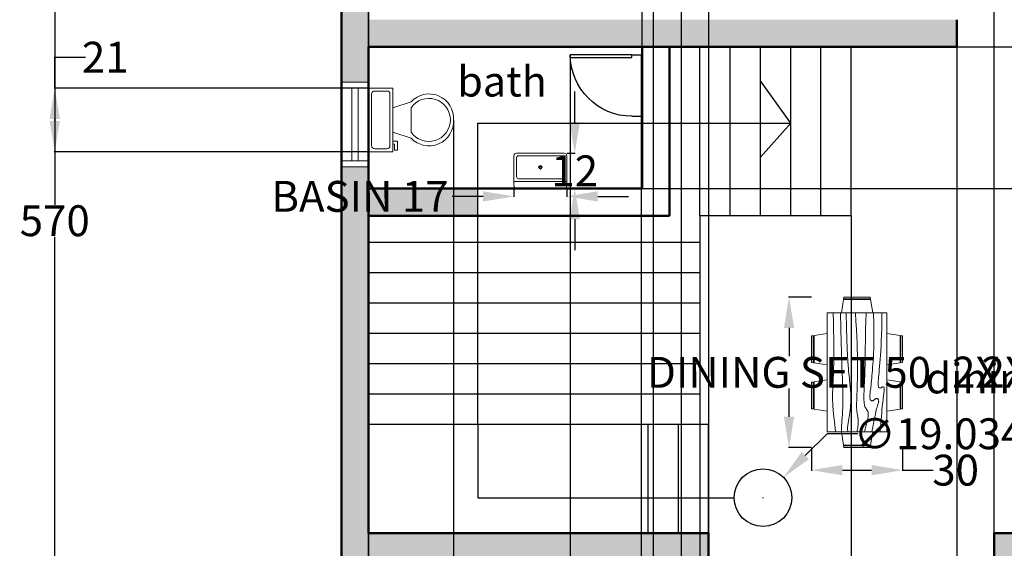
# Model space of a CAD drawing. Units: inches. Extents: x 12496 to 13538, y 6171 to 6892.
# Tile 2 of 6: x 12516 to 12841, y 6398 to 6572. Entities that reach past the tile are written whole.
import ezdxf

# ---------------------------------------------------------------- set-up
doc = ezdxf.new("R2010")
doc.units = ezdxf.units.IN
doc.header["$MEASUREMENT"] = 0
for name, color, linetype, lineweight in [('A-ANNO-DIMS', 2, 'Continuous', 18), ('A-AREA-IDEN', 7, 'Continuous', 25), ('A-DOOR', 3, 'Continuous', 25), ('A-FLOR-FIXT', 9, 'Continuous', 18), ('A-FLOR-STRS', 7, 'Continuous', 25), ('A-FURN', 8, 'Continuous', 18), ('A-GLAZ', 4, 'Continuous', 18), ('A-WALL', 7, 'Continuous', 50)]:
    doc.layers.add(name, color=color, linetype=linetype, lineweight=lineweight)
doc.layers.add('A-WALL-PATT', color=18, linetype='Continuous', lineweight=13, true_color=0x000000)
doc.styles.get("Standard").update_dxf_attribs({"font": 'arial.ttf'})
doc.dimstyles.get("Standard").update_dxf_attribs({"dimtxt": 10.18, "dimasz": 10.18, "dimexe": 0.18, "dimexo": 0.0625, "dimgap": 0.09, "dimtad": 0, "dimtih": 1, "dimtoh": 1, "dimdec": 0, "dimzin": 0, "dimdsep": 46, "dimlunit": 3, "dimtxsty": 'Standard', "dimcen": 0.09, "dimadec": 0, "dimazin": 0, "dimtfac": 1, "dimtdec": 0, "dimtofl": 0, "dimtmove": 0, "dimatfit": 3, "dimfxl": 1, "dimtolj": 1, "dimtzin": 0, "dimarcsym": 0})

# ---------------------------------------------------------------- blocks, each defined once
blk = doc.blocks.new('*U2')
for p, q in [((0, 0), (0, -6)), ((40, 0), (40, -6))]:
    blk.add_line(p, q)
blk.add_lwpolyline([(0, 0), (0, 40), (1.75, 40), (1.75, 0)], close=True)
blk.add_arc((0, 0), 40, 0, 90)
blk = doc.blocks.new('Dining Set - 36 x 72 in.')
for p, q in [((-22.2343, 26.00059), (-23.4847, 17.99762)), ((-22.2304, 26), (-5.7608, 26)), ((-22, 27.5), (-22.1562, 26.50042)), ((-5.8416, 26.5), (-22.1534, 26.5)), ((-22, 27.5), (-6, 27.5)), ((-5.8437, 26.49966), (-6, 27.5)), ((-4.5152, 17.99762), (-5.7655, 25.99926)), ((5.7657, 26.00059), (4.5153, 17.99762)), ((5.7696, 26), (22.2392, 26)), ((6, 27.5), (5.8438, 26.50042)), ((22.1584, 26.5), (5.8466, 26.5)), ((6, 27.5), (22, 27.5)), ((22.1563, 26.49966), (22, 27.5)), ((23.4848, 17.99762), (22.2345, 25.99926)), ((36, 18), (-36, 18)), ((-36, 18), (-36, -18)), ((36, -18), (36, 18)), ((-45.5, 8), (-44.5004, 8.15617)), ((-45.5, 8), (-45.5, -8)), ((-44.5, -8.15843), (-44.5, 8.15338)), ((-44.0006, 8.23428), (-35.9976, 9.48474)), ((-44, 8.23041), (-44, -8.23915)), ((44.0006, 8.23428), (35.9976, 9.48474)), ((44, 8.23041), (44, -8.23915)), ((44.5, -8.15843), (44.5, 8.15338)), ((45.5, 8), (44.5005, 8.15617)), ((45.5, 8), (45.5, -8)), ((-44.4997, -8.15631), (-45.5, -8)), ((-35.9976, -9.48476), (-43.9993, -8.2345)), ((35.9976, -9.48476), (43.9993, -8.2345)), ((44.4997, -8.15631), (45.5, -8)), ((-36, -18), (36, -18)), ((-22.2343, -26.0006), (-23.4847, -17.99762)), ((-4.5152, -17.99762), (-5.7655, -25.99928)), ((5.7657, -26.0006), (4.5153, -17.99762)), ((23.4848, -17.99762), (22.2345, -25.99928)), ((-22.2304, -26), (-5.7608, -26)), ((-22, -27.5), (-22.1562, -26.50044)), ((-5.8416, -26.5), (-22.1534, -26.5)), ((-22, -27.5), (-6, -27.5)), ((-5.8437, -26.49967), (-6, -27.5)), ((5.7696, -26), (22.2392, -26)), ((6, -27.5), (5.8438, -26.50044)), ((22.1584, -26.5), (5.8466, -26.5)), ((6, -27.5), (22, -27.5)), ((22.1563, -26.49967), (22, -27.5))]:
    blk.add_line(p, q)
for points in [[(-36, 15), (-31.1772, 14.97754), (-26.8079, 14.91406), (-22.8538, 14.81543), (-19.276, 14.6875), (-16.0362, 14.53613), (-13.0957, 14.36718), (-10.4159, 14.18652), (-7.9583, 14), (-5.6904, 13.81315), (-3.6035, 13.63021), (-1.6954, 13.45508), (0.0365, 13.29166), (1.5945, 13.14388), (2.9811, 13.01562), (4.1988, 12.9108), (5.25, 12.83333), (6.1393, 12.78613), (6.8802, 12.76823), (7.4883, 12.77767), (7.9792, 12.8125), (8.3685, 12.87077), (8.6719, 12.95052), (8.9049, 13.0498), (9.0833, 13.16666), (9.2205, 13.29899), (9.3216, 13.44401), (9.3895, 13.59879), (9.4271, 13.76041), (9.4373, 13.92594), (9.4232, 14.09245), (9.3875, 14.257), (9.3333, 14.41666), (9.2638, 14.56917), (9.1836, 14.71484), (9.0975, 14.85465), (9.0104, 14.98958), (8.9272, 15.1206), (8.8529, 15.2487), (8.7922, 15.37483), (8.75, 15.5), (8.7305, 15.62467), (8.7344, 15.74739), (8.7617, 15.86621), (8.8125, 15.97916), (8.8867, 16.08431), (8.9844, 16.17968), (9.1055, 16.26334), (9.25, 16.33333), (9.4189, 16.38802), (9.6172, 16.42708), (9.8506, 16.45052), (10.125, 16.45833), (10.4463, 16.45052), (10.8203, 16.42708), (11.2529, 16.38802), (11.75, 16.33333), (12.3184, 16.26318), (12.9694, 16.17838), (13.7151, 16.07991), (14.5677, 15.96875), (15.5395, 15.84586), (16.6426, 15.71224), (17.8893, 15.56884), (19.2917, 15.41666), (20.859, 15.25667), (22.5879, 15.08984), (24.4721, 14.91715), (26.5052, 14.73958), (28.6809, 14.5581), (30.9929, 14.3737), (33.4347, 14.18733), (36, 14)], [(-36, 10), (-28.9766, 10.14274), (-23.1725, 10.20442), (-18.4241, 10.19775), (-14.5677, 10.13541), (-11.4399, 10.03011), (-8.877, 9.89453), (-6.7154, 9.74137), (-4.7917, 9.58333), (-2.9698, 9.43082), (-1.2246, 9.28515), (0.4415, 9.14534), (2.026, 9.01041), (3.5266, 8.87939), (4.9408, 8.7513), (6.266, 8.62516), (7.5, 8.5), (8.6411, 8.37549), (9.6914, 8.2539), (10.6538, 8.13818), (11.5312, 8.03125), (12.3267, 7.93603), (13.043, 7.85547), (13.6831, 7.79248), (14.25, 7.75), (14.7471, 7.7303), (15.1797, 7.73307), (15.5537, 7.75732), (15.875, 7.80208), (16.1494, 7.86637), (16.3828, 7.94922), (16.5811, 8.04964), (16.75, 8.16666), (16.8944, 8.29915), (17.0143, 8.44531), (17.1089, 8.60319), (17.1771, 8.77083), (17.218, 8.94629), (17.2305, 9.1276), (17.2137, 9.31282), (17.1667, 9.5), (17.0895, 9.6875), (16.987, 9.875), (16.8649, 10.0625), (16.7292, 10.25), (16.5856, 10.4375), (16.4401, 10.625), (16.2985, 10.8125), (16.1667, 11), (16.05, 11.18733), (15.9518, 11.3737), (15.8752, 11.5581), (15.8229, 11.73958), (15.798, 11.91715), (15.8034, 12.08984), (15.842, 12.25667), (15.9167, 12.41666), (16.0295, 12.56836), (16.1784, 12.70833), (16.3605, 12.83268), (16.5729, 12.9375), (16.8127, 13.01888), (17.0768, 13.07291), (17.3625, 13.0957), (17.6667, 13.08333), (17.9894, 13.03312), (18.3418, 12.94726), (18.7382, 12.82918), (19.1927, 12.68229), (19.7195, 12.51001), (20.3327, 12.31575), (21.0465, 12.10294), (21.875, 11.875), (22.8357, 11.63354), (23.959, 11.37304), (25.2786, 11.08618), (26.8282, 10.76562), (28.6414, 10.40405), (30.752, 9.99414), (33.1936, 9.52856), (36, 9)], [(-36, 5.5), (-30.7157, 5.3348), (-26.069, 5.20963), (-21.9946, 5.11767), (-18.4271, 5.05208), (-15.3009, 5.00602), (-12.5508, 4.97265), (-10.1112, 4.94515), (-7.9167, 4.91666), (-5.909, 4.88167), (-4.0586, 4.83984), (-2.3429, 4.79215), (-0.7396, 4.73958), (0.7739, 4.6831), (2.22, 4.6237), (3.6213, 4.56233), (5, 4.5), (6.373, 4.43782), (7.7344, 4.3776), (9.0723, 4.32129), (10.375, 4.27083), (11.6309, 4.22819), (12.8281, 4.19531), (13.9551, 4.17415), (15, 4.16666), (15.954, 4.17448), (16.819, 4.19791), (17.6001, 4.23698), (18.3021, 4.29166), (18.9299, 4.36198), (19.4883, 4.44791), (19.9823, 4.54948), (20.4167, 4.66666), (20.7969, 4.79899), (21.1302, 4.94401), (21.4245, 5.09879), (21.6875, 5.26041), (21.9271, 5.42594), (22.1511, 5.59245), (22.3672, 5.757), (22.5834, 5.91666), (22.8065, 6.06868), (23.0404, 6.21093), (23.2879, 6.34147), (23.5521, 6.45833), (23.8358, 6.55957), (24.142, 6.64323), (24.4735, 6.70735), (24.8334, 6.75), (25.2235, 6.76969), (25.642, 6.76692), (26.0858, 6.74267), (26.5521, 6.69791), (27.0379, 6.63362), (27.5404, 6.55078), (28.0565, 6.45036), (28.5834, 6.33333), (29.1242, 6.19987), (29.7071, 6.04687), (30.3661, 5.87044), (31.1354, 5.66666), (32.0493, 5.43164), (33.142, 5.16146), (34.4475, 4.85221), (36, 4.5)], [(-36, -1), (-30.7915, -0.6591), (-26.0195, -0.38216), (-21.6519, -0.16284), (-17.6563, 0.00521), (-14.0005, 0.12833), (-10.6523, 0.21289), (-7.5796, 0.26522), (-4.75, 0.29166), (-2.134, 0.29793), (0.2878, 0.28711), (2.5317, 0.26163), (4.6146, 0.22396), (6.5529, 0.17651), (8.3633, 0.12174), (10.0623, 0.06209), (11.6667, 0), (13.1899, -0.06201), (14.6341, -0.1211), (15.9982, -0.17432), (17.2813, -0.21875), (18.4823, -0.25147), (19.6003, -0.26953), (20.6343, -0.27002), (21.5834, -0.25), (22.4481, -0.20768), (23.2357, -0.14584), (23.9549, -0.06836), (24.6146, 0.02083), (25.2235, 0.11784), (25.7904, 0.21875), (26.3241, 0.31966), (26.8334, 0.41666), (27.3265, 0.50618), (27.8099, 0.58593), (28.2894, 0.65397), (28.7709, 0.70833), (29.2601, 0.74707), (29.763, 0.76823), (30.2855, 0.76985), (30.8334, 0.75), (31.4088, 0.70784), (31.9994, 0.64713), (32.589, 0.57275), (33.1615, 0.48958), (33.7008, 0.4025), (34.1908, 0.3164), (34.6153, 0.23616), (34.9584, 0.16666), (35.2099, 0.11165), (35.3848, 0.07031), (35.504, 0.04069), (35.5886, 0.02083), (35.6594, 0.00879), (35.7377, 0.0026), (35.8442, 0.00032), (36, 0)], [(-36, -6.5), (-27.1843, -6.31267), (-20.084, -6.1263), (-14.469, -5.9419), (-10.1094, -5.76042), (-6.7752, -5.58285), (-4.2363, -5.41016), (-2.2629, -5.24333), (-0.625, -5.08334), (0.8708, -4.93099), (2.2715, -4.78646), (3.5872, -4.64974), (4.8281, -4.52084), (6.0046, -4.39974), (7.127, -4.28646), (8.2053, -4.18099), (9.25, -4.08334), (10.2705, -3.99382), (11.2734, -3.91407), (12.2647, -3.84603), (13.25, -3.79167), (14.2354, -3.75293), (15.2266, -3.73177), (16.2295, -3.73015), (17.25, -3.75), (18.2912, -3.79248), (19.3451, -3.85547), (20.4009, -3.93604), (21.4479, -4.03125), (22.4754, -4.13819), (23.4727, -4.25391), (24.4289, -4.37549), (25.3334, -4.5), (26.1785, -4.62492), (26.9694, -4.74935), (27.7145, -4.87281), (28.4219, -4.99479), (29.1, -5.11483), (29.7572, -5.23242), (30.4016, -5.34709), (31.0417, -5.45834), (31.6837, -5.56437), (32.3262, -5.65821), (32.9658, -5.73153), (33.599, -5.77604), (34.2224, -5.78345), (34.8327, -5.74545), (35.4264, -5.65373), (36, -5.5)], [(-36, -10), (-26.4022, -9.81299), (-18.4675, -9.62891), (-11.9839, -9.45069), (-6.7396, -9.28125), (-2.5226, -9.12354), (0.8789, -8.98047), (3.6769, -8.85498), (6.0833, -8.75), (8.2767, -8.66765), (10.3021, -8.60677), (12.1712, -8.56543), (13.8958, -8.54167), (15.4876, -8.53353), (16.9583, -8.53907), (18.3197, -8.55632), (19.5834, -8.58334), (20.7616, -8.61841), (21.8685, -8.66081), (22.9188, -8.71004), (23.9271, -8.76563), (24.9081, -8.82707), (25.8763, -8.89388), (26.8465, -8.96558), (27.8334, -9.04167), (28.8474, -9.12118), (29.8828, -9.20117), (30.93, -9.27824), (31.9792, -9.34896), (33.0205, -9.40991), (34.0443, -9.45768), (35.0407, -9.48885), (36, -9.5)], [(-36, -14.5), (-30.0881, -14.33513), (-25.0332, -14.21224), (-20.7312, -14.12647), (-17.0781, -14.07292), (-13.97, -14.04671), (-11.3027, -14.04297), (-8.9724, -14.05681), (-6.875, -14.08334), (-4.9224, -14.11833), (-3.0905, -14.16016), (-1.3709, -14.20785), (0.2448, -14.26042), (1.7647, -14.3169), (3.1973, -14.3763), (4.5507, -14.43767), (5.8333, -14.5), (7.0554, -14.5621), (8.235, -14.62175), (9.3922, -14.67652), (10.5469, -14.72396), (11.7192, -14.76164), (12.929, -14.78711), (14.1965, -14.79794), (15.5417, -14.79167), (16.9933, -14.76424), (18.6152, -14.70508), (20.4804, -14.60197), (22.6615, -14.44271), (25.2312, -14.21509), (28.2624, -13.9069), (31.8277, -13.50594), (36, -13)]]:
    blk.add_lwpolyline(points)
blk = doc.blocks.new('*U16')
for p, q in [((9.5, -6), (9.5, -2)), ((-10, -8.5), (-8, -8.5)), ((-10, -9.5), (-10, -8.5)), ((-7, -9.5), (-10, -9.5)), ((-8, -8.5), (-8, -8)), ((-7, -8), (-7, -9.5)), ((-4, -8), (-6, -14)), ((4, -8), (6, -14)), ((4, -14), (-4, -14))]:
    blk.add_line(p, q)
blk.add_lwpolyline([(10.5, -8), (10.5, 0), (-10.5, 0), (-10.5, -8)], close=True)
for points in [[(-9.5, -2), (-9.5, -6)], [(8.5, -1), (-8.5, -1)], [(-8.5, -7), (8.5, -7)]]:
    blk.add_lwpolyline(points)
for centre, radius, start, end in [((-8.625, -1.875), 0.8839, 81.8699, 188.1301), ((8.625, -1.875), 0.8839, 351.8699, 98.1301), ((-8.625, -6.125), 0.8839, 171.869898, 278.1301), ((8.625, -6.125), 0.8839, 261.8699, 8.1301), ((-0.4772, -19.9188), 8.0953, 133.01722, 273.38), ((0.0374, -19.8731), 7.127, 124.50543, 269.7), ((-0.0373, -19.8731), 7.127, 270.3, 55.4946), ((0.4773, -19.9188), 8.0953, 266.62, 46.9828)]:
    blk.add_arc(centre, radius, start, end)
blk = doc.blocks.new('Sink-single - 30 in top')
blk.add_line((-15, -3.999996), (15, -3.999996))
for points in [[(-13.5, 0), (13.5, 0)], [(-15, -18.499996), (-15, -1.5)], [(-12.5, -5.499996), (12.5, -5.499996)], [(15, -1.5), (15, -18.499996)], [(-13.5, -17.499996), (-13.5, -6.499996)], [(13.5, -6.499996), (13.5, -17.499996)], [(13.5, -19.999996), (-13.5, -19.999996)], [(12.5, -18.499996), (-12.5, -18.499996)]]:
    blk.add_lwpolyline(points)
for radius in [1, 0.5]:
    blk.add_circle((0, -11.999996), radius)
for centre, radius, start, end in [((-13.5, -1.5), 1.5, 90, 180), ((-12.5, -6.499996), 1, 90, 180), ((12.5, -6.499996), 1, 0, 90), ((13.5, -1.5), 1.5, 0, 90), ((-13.5, -18.499996), 1.5, 180, 270), ((-12.5, -17.499996), 1, 180, 270), ((12.5, -17.499996), 1, 270, 0), ((13.5, -18.499996), 1.5, 270, 0)]:
    blk.add_arc(centre, radius, start, end)
blk = doc.blocks.new('WIN-24IN')
for p, q in [((0, 0), (0, 9)), ((2, 0), (2, 9)), ((26, 0), (26, 9)), ((28, 0), (28, 9)), ((2, 5.5), (26, 5.5)), ((2, 3.5), (26, 3.5))]:
    blk.add_line(p, q)
blk = doc.blocks.new('*D37')
at = {"layer": 'A-ANNO-DIMS', "color": 0, "lineweight": -2, "transparency": 16777216}
for p, q in [((12679.14, 6516.47), (12679.14, 6513.74)), ((12696.58, 6516.47), (12696.58, 6513.74)), ((12668.96, 6513.92), (12658.78, 6513.92)), ((12706.76, 6513.92), (12716.94, 6513.92))]:
    blk.add_line(p, q, dxfattribs=at)
at = {"layer": 'A-ANNO-DIMS', "color": 0, "transparency": 16777216}
for points in [[(12668.96, 6515.62), (12668.96, 6512.22), (12679.14, 6513.92)], [(12706.76, 6515.62), (12706.76, 6512.22), (12696.58, 6513.92)]]:
    blk.add_solid(points, dxfattribs=at)
at = {"layer": 'Defpoints', "color": 0, "transparency": 16777216}
for p in [(12679.14, 6516.54), (12696.58, 6516.54), (12679.14, 6513.92)]:
    blk.add_point(p, dxfattribs=at)
at = {"layer": 'A-ANNO-DIMS', "color": 0, "transparency": 16777216, "insert": (12628.31, 6513.92), "char_height": 10.18, "attachment_point": 5}
blk.add_mtext('\\A1;BASIN 17', dxfattribs=at)
blk = doc.blocks.new('*D38')
at = {"layer": 'A-ANNO-DIMS', "color": 0, "lineweight": -2, "transparency": 16777216}
for p, q in [((12699.19, 6538.34), (12699.19, 6548.52)), ((12696.64, 6528.16), (12699.37, 6528.16)), ((12696.64, 6516.54), (12699.37, 6516.54)), ((12699.19, 6506.36), (12699.19, 6496.18))]:
    blk.add_line(p, q, dxfattribs=at)
at = {"layer": 'A-ANNO-DIMS', "color": 0, "transparency": 16777216}
for points in [[(12697.5, 6538.34), (12700.89, 6538.34), (12699.19, 6528.16)], [(12697.5, 6506.36), (12700.89, 6506.36), (12699.19, 6516.54)]]:
    blk.add_solid(points, dxfattribs=at)
at = {"layer": 'Defpoints', "color": 0, "transparency": 16777216}
for p in [(12696.58, 6528.16), (12696.58, 6516.54), (12699.19, 6516.54)]:
    blk.add_point(p, dxfattribs=at)
at = {"layer": 'A-ANNO-DIMS', "color": 0, "transparency": 16777216, "insert": (12699.19, 6522.35), "char_height": 10.18, "attachment_point": 5}
blk.add_mtext('\\A1;12', dxfattribs=at)
blk = doc.blocks.new('*D51')
at = {"layer": 'A-ANNO-DIMS', "color": 0, "lineweight": -2, "transparency": 16777216}
for p, q in [((12777.29, 6480.69), (12769.73, 6480.69)), ((12769.91, 6470.51), (12769.91, 6461.22)), ((12769.91, 6441.23), (12769.91, 6450.51)), ((12777.29, 6431.05), (12769.73, 6431.05))]:
    blk.add_line(p, q, dxfattribs=at)
at = {"layer": 'A-ANNO-DIMS', "color": 0, "transparency": 16777216}
for points in [[(12768.21, 6470.51), (12771.61, 6470.51), (12769.91, 6480.69)], [(12768.21, 6441.23), (12771.61, 6441.23), (12769.91, 6431.05)]]:
    blk.add_solid(points, dxfattribs=at)
at = {"layer": 'Defpoints', "color": 0, "transparency": 16777216}
for p in [(12777.35, 6480.69), (12769.91, 6431.05), (12777.35, 6431.05)]:
    blk.add_point(p, dxfattribs=at)
at = {"layer": 'A-ANNO-DIMS', "color": 0, "transparency": 16777216, "insert": (12769.91, 6455.87), "char_height": 10.18, "attachment_point": 5}
blk.add_mtext('\\A1;DINING SET 50', dxfattribs=at)
blk = doc.blocks.new('*D52')
at = {"layer": 'A-ANNO-DIMS', "color": 0, "lineweight": -2, "transparency": 16777216}
for p, q in [((12777.35, 6430.99), (12777.35, 6423.43)), ((12807.35, 6430.99), (12807.35, 6423.43)), ((12787.53, 6423.61), (12797.17, 6423.61)), ((12807.35, 6423.61), (12817.53, 6423.61))]:
    blk.add_line(p, q, dxfattribs=at)
at = {"layer": 'A-ANNO-DIMS', "color": 0, "transparency": 16777216}
for points in [[(12787.53, 6425.3), (12787.53, 6421.91), (12777.35, 6423.61)], [(12797.17, 6425.3), (12797.17, 6421.91), (12807.35, 6423.61)]]:
    blk.add_solid(points, dxfattribs=at)
at = {"layer": 'Defpoints', "color": 0, "transparency": 16777216}
for p in [(12777.35, 6431.05), (12807.35, 6431.05), (12807.35, 6423.61)]:
    blk.add_point(p, dxfattribs=at)
at = {"layer": 'A-ANNO-DIMS', "color": 0, "transparency": 16777216, "insert": (12824.89, 6423.61), "char_height": 10.18, "attachment_point": 5}
blk.add_mtext('\\A1;30', dxfattribs=at)
blk = doc.blocks.new('*D60')
at = {"layer": 'A-ANNO-DIMS', "color": 0, "lineweight": -2, "transparency": 16777216}
for p, q in [((12622.11, 6790.89), (12527.4, 6790.89)), ((12527.58, 6780.71), (12527.58, 6511.18)), ((12527.58, 6231.07), (12527.58, 6500.61)), ((12622.11, 6220.89), (12527.4, 6220.89))]:
    blk.add_line(p, q, dxfattribs=at)
at = {"layer": 'A-ANNO-DIMS', "color": 0, "transparency": 16777216}
for points in [[(12525.88, 6780.71), (12529.28, 6780.71), (12527.58, 6790.89)], [(12525.88, 6231.07), (12529.28, 6231.07), (12527.58, 6220.89)]]:
    blk.add_solid(points, dxfattribs=at)
at = {"layer": 'Defpoints', "color": 0, "transparency": 16777216}
for p in [(12527.58, 6790.89), (12622.17, 6790.89), (12622.17, 6220.89)]:
    blk.add_point(p, dxfattribs=at)
at = {"layer": 'A-ANNO-DIMS', "color": 0, "transparency": 16777216, "insert": (12527.58, 6505.89), "char_height": 10.18, "attachment_point": 5}
blk.add_mtext('\\A1;570', dxfattribs=at)
blk = doc.blocks.new('*D65')
at = {"layer": 'A-ANNO-DIMS', "color": 0, "lineweight": -2, "transparency": 16777216}
for p, q in [((12631.17, 6229.96), (12631.17, 6885.67)), ((12641.35, 6885.49), (12713.08, 6885.49)), ((12827.42, 6885.49), (12755.7, 6885.49)), ((12837.6, 6229.96), (12837.6, 6885.67))]:
    blk.add_line(p, q, dxfattribs=at)
at = {"layer": 'A-ANNO-DIMS', "color": 0, "transparency": 16777216}
for points in [[(12641.35, 6887.18), (12641.35, 6883.79), (12631.17, 6885.49)], [(12827.42, 6887.18), (12827.42, 6883.79), (12837.6, 6885.49)]]:
    blk.add_solid(points, dxfattribs=at)
at = {"layer": 'Defpoints', "color": 0, "transparency": 16777216}
for p in [(12837.6, 6885.49), (12631.17, 6229.89), (12837.6, 6229.89)]:
    blk.add_point(p, dxfattribs=at)
at = {"layer": 'A-ANNO-DIMS', "color": 0, "transparency": 16777216, "insert": (12734.39, 6885.49), "char_height": 10.18, "attachment_point": 5}
blk.add_mtext('\\A1;206.43', dxfattribs=at)
blk = doc.blocks.new('*D73')
at = {"layer": 'A-ANNO-DIMS', "color": 0, "lineweight": -2, "transparency": 16777216}
for p, q in [((12631.17, 6393.87), (12631.17, 6885.67)), ((12641.35, 6885.49), (12663.02, 6885.49)), ((12724.21, 6885.49), (12702.54, 6885.49)), ((12734.39, 6393.87), (12734.39, 6885.67))]:
    blk.add_line(p, q, dxfattribs=at)
at = {"layer": 'A-ANNO-DIMS', "color": 0, "transparency": 16777216}
for points in [[(12641.35, 6887.18), (12641.35, 6883.79), (12631.17, 6885.49)], [(12724.21, 6887.18), (12724.21, 6883.79), (12734.39, 6885.49)]]:
    blk.add_solid(points, dxfattribs=at)
at = {"layer": 'Defpoints', "color": 0, "transparency": 16777216}
for p in [(12734.39, 6885.49), (12631.17, 6393.81), (12734.39, 6393.81)]:
    blk.add_point(p, dxfattribs=at)
at = {"layer": 'A-ANNO-DIMS', "color": 0, "transparency": 16777216, "insert": (12682.78, 6885.49), "char_height": 10.18, "attachment_point": 5}
blk.add_mtext('\\A1;103.21', dxfattribs=at)
blk = doc.blocks.new('*D75')
at = {"layer": 'A-ANNO-DIMS', "color": 0, "lineweight": -2, "transparency": 16777216}
for p, q in [((12631.17, 6563.27), (12631.17, 6885.67)), ((12641.35, 6885.49), (12659.04, 6885.49)), ((12711.27, 6885.49), (12693.59, 6885.49)), ((12721.45, 6563.27), (12721.45, 6885.67))]:
    blk.add_line(p, q, dxfattribs=at)
at = {"layer": 'A-ANNO-DIMS', "color": 0, "transparency": 16777216}
for points in [[(12641.35, 6887.18), (12641.35, 6883.79), (12631.17, 6885.49)], [(12711.27, 6887.18), (12711.27, 6883.79), (12721.45, 6885.49)]]:
    blk.add_solid(points, dxfattribs=at)
at = {"layer": 'Defpoints', "color": 0, "transparency": 16777216}
for p in [(12721.45, 6885.49), (12631.17, 6563.2), (12721.45, 6563.2)]:
    blk.add_point(p, dxfattribs=at)
at = {"layer": 'A-ANNO-DIMS', "color": 0, "transparency": 16777216, "insert": (12676.31, 6885.49), "char_height": 10.18, "attachment_point": 5}
blk.add_mtext('\\A1;90.28', dxfattribs=at)
blk = doc.blocks.new('*D76')
at = {"layer": 'A-ANNO-DIMS', "color": 0, "lineweight": -2, "transparency": 16777216}
for p, q in [((12721.51, 6563.2), (13486.8, 6563.2)), ((13486.62, 6553.02), (13486.62, 6545.16)), ((13486.62, 6526.72), (13486.62, 6534.58)), ((12721.51, 6516.54), (13486.8, 6516.54))]:
    blk.add_line(p, q, dxfattribs=at)
at = {"layer": 'A-ANNO-DIMS', "color": 0, "transparency": 16777216}
for points in [[(13484.92, 6553.02), (13488.32, 6553.02), (13486.62, 6563.2)], [(13484.92, 6526.72), (13488.32, 6526.72), (13486.62, 6516.54)]]:
    blk.add_solid(points, dxfattribs=at)
at = {"layer": 'Defpoints', "color": 0, "transparency": 16777216}
for p in [(12721.45, 6563.2), (13486.62, 6563.2), (12721.45, 6516.54)]:
    blk.add_point(p, dxfattribs=at)
at = {"layer": 'A-ANNO-DIMS', "color": 0, "transparency": 16777216, "insert": (13486.62, 6539.87), "char_height": 10.18, "attachment_point": 5}
blk.add_mtext('\\A1;46.67', dxfattribs=at)
blk = doc.blocks.new('*D77')
at = {"layer": 'A-ANNO-DIMS', "color": 0, "lineweight": -2, "transparency": 16777216}
for p, q in [((12721.09, 6560.6), (12721.09, 6177.12)), ((12697.73, 6559.71), (12697.73, 6177.12)), ((12707.91, 6177.3), (12710.91, 6177.3)), ((12721.09, 6177.3), (12731.27, 6177.3))]:
    blk.add_line(p, q, dxfattribs=at)
at = {"layer": 'A-ANNO-DIMS', "color": 0, "transparency": 16777216}
for points in [[(12707.91, 6179), (12707.91, 6175.6), (12697.73, 6177.3)], [(12710.91, 6179), (12710.91, 6175.6), (12721.09, 6177.3)]]:
    blk.add_solid(points, dxfattribs=at)
at = {"layer": 'Defpoints', "color": 0, "transparency": 16777216}
for p in [(12721.09, 6560.66), (12697.73, 6559.77), (12721.09, 6177.3)]:
    blk.add_point(p, dxfattribs=at)
at = {"layer": 'A-ANNO-DIMS', "color": 0, "transparency": 16777216, "insert": (12752.61, 6177.3), "char_height": 10.18, "attachment_point": 5}
blk.add_mtext('\\A1;23.355', dxfattribs=at)
blk = doc.blocks.new('*D78')
at = {"layer": 'A-ANNO-DIMS', "color": 0, "lineweight": -2, "transparency": 16777216}
for p, q in [((12527.58, 6549.65), (12527.58, 6559.83)), ((12527.58, 6559.83), (12537.76, 6559.83)), ((12631.11, 6549.65), (12527.4, 6549.65)), ((12527.58, 6538.83), (12527.58, 6539.47)), ((12631.11, 6528.65), (12527.4, 6528.65))]:
    blk.add_line(p, q, dxfattribs=at)
at = {"layer": 'A-ANNO-DIMS', "color": 0, "transparency": 16777216}
for points in [[(12525.88, 6539.47), (12529.28, 6539.47), (12527.58, 6549.65)], [(12525.88, 6538.83), (12529.28, 6538.83), (12527.58, 6528.65)]]:
    blk.add_solid(points, dxfattribs=at)
at = {"layer": 'Defpoints', "color": 0, "transparency": 16777216}
for p in [(12527.58, 6549.65), (12631.17, 6549.65), (12631.17, 6528.65)]:
    blk.add_point(p, dxfattribs=at)
at = {"layer": 'A-ANNO-DIMS', "color": 0, "transparency": 16777216, "insert": (12544.25, 6559.83), "char_height": 10.18, "attachment_point": 5}
blk.add_mtext('\\A1;21', dxfattribs=at)
blk = doc.blocks.new('*D79')
at = {"layer": 'A-ANNO-DIMS', "color": 0, "lineweight": -2, "transparency": 16777216}
for p, q in [((12659.17, 6539.09), (12659.17, 6177.12)), ((12631.17, 6528.59), (12631.17, 6177.12)), ((12641.35, 6177.3), (12648.99, 6177.3)), ((12659.17, 6177.3), (12669.35, 6177.3))]:
    blk.add_line(p, q, dxfattribs=at)
at = {"layer": 'A-ANNO-DIMS', "color": 0, "transparency": 16777216}
for points in [[(12641.35, 6179), (12641.35, 6175.6), (12631.17, 6177.3)], [(12648.99, 6179), (12648.99, 6175.6), (12659.17, 6177.3)]]:
    blk.add_solid(points, dxfattribs=at)
at = {"layer": 'Defpoints', "color": 0, "transparency": 16777216}
for p in [(12659.17, 6539.15), (12631.17, 6528.65), (12659.17, 6177.3)]:
    blk.add_point(p, dxfattribs=at)
at = {"layer": 'A-ANNO-DIMS', "color": 0, "transparency": 16777216, "insert": (12676.83, 6177.3), "char_height": 10.18, "attachment_point": 5}
blk.add_mtext('\\A1;28', dxfattribs=at)
blk = doc.blocks.new('*D80')
at = {"layer": 'A-ANNO-DIMS', "color": 0, "lineweight": -2, "transparency": 16777216}
for p, q in [((12631.17, 6781.83), (12631.17, 6177.12)), ((12725.12, 6781.83), (12725.12, 6177.12)), ((12641.35, 6177.3), (12660.84, 6177.3)), ((12714.94, 6177.3), (12695.45, 6177.3))]:
    blk.add_line(p, q, dxfattribs=at)
at = {"layer": 'A-ANNO-DIMS', "color": 0, "transparency": 16777216}
for points in [[(12641.35, 6179), (12641.35, 6175.6), (12631.17, 6177.3)], [(12714.94, 6179), (12714.94, 6175.6), (12725.12, 6177.3)]]:
    blk.add_solid(points, dxfattribs=at)
at = {"layer": 'Defpoints', "color": 0, "transparency": 16777216}
for p in [(12631.17, 6781.89), (12725.12, 6781.89), (12725.12, 6177.3)]:
    blk.add_point(p, dxfattribs=at)
at = {"layer": 'A-ANNO-DIMS', "color": 0, "transparency": 16777216, "insert": (12678.15, 6177.3), "char_height": 10.18, "attachment_point": 5}
blk.add_mtext('\\A1;93.95', dxfattribs=at)
blk = doc.blocks.new('*D85')
at = {"layer": 'A-ANNO-DIMS', "color": 0, "lineweight": -2, "transparency": 16777216}
for p, q in [((12743.39, 6402.87), (12743.39, 6885.67)), ((12753.57, 6885.49), (12774.21, 6885.49)), ((12827.42, 6885.49), (12806.78, 6885.49)), ((12837.6, 6402.87), (12837.6, 6885.67))]:
    blk.add_line(p, q, dxfattribs=at)
at = {"layer": 'A-ANNO-DIMS', "color": 0, "transparency": 16777216}
for points in [[(12753.57, 6887.18), (12753.57, 6883.79), (12743.39, 6885.49)], [(12827.42, 6887.18), (12827.42, 6883.79), (12837.6, 6885.49)]]:
    blk.add_solid(points, dxfattribs=at)
at = {"layer": 'Defpoints', "color": 0, "transparency": 16777216}
for p in [(12837.6, 6885.49), (12743.39, 6402.81), (12837.6, 6402.81)]:
    blk.add_point(p, dxfattribs=at)
at = {"layer": 'A-ANNO-DIMS', "color": 0, "transparency": 16777216, "insert": (12790.5, 6885.49), "char_height": 10.18, "attachment_point": 5}
blk.add_mtext('\\A1;94.21', dxfattribs=at)
blk = doc.blocks.new('*D86')
at = {"layer": 'A-ANNO-DIMS', "color": 0, "lineweight": -2, "transparency": 16777216}
for p, q in [((12740.45, 6507.47), (12740.45, 6177.12)), ((12790.45, 6507.47), (12790.45, 6177.12)), ((12750.63, 6177.3), (12758.09, 6177.3)), ((12780.27, 6177.3), (12772.81, 6177.3))]:
    blk.add_line(p, q, dxfattribs=at)
at = {"layer": 'A-ANNO-DIMS', "color": 0, "transparency": 16777216}
for points in [[(12750.63, 6179), (12750.63, 6175.6), (12740.45, 6177.3)], [(12780.27, 6179), (12780.27, 6175.6), (12790.45, 6177.3)]]:
    blk.add_solid(points, dxfattribs=at)
at = {"layer": 'Defpoints', "color": 0, "transparency": 16777216}
for p in [(12740.45, 6507.54), (12790.45, 6507.54), (12790.45, 6177.3)]:
    blk.add_point(p, dxfattribs=at)
at = {"layer": 'A-ANNO-DIMS', "color": 0, "transparency": 16777216, "insert": (12765.45, 6177.3), "char_height": 10.18, "attachment_point": 5}
blk.add_mtext('\\A1;50', dxfattribs=at)
blk = doc.blocks.new('*D87')
at = {"layer": 'A-ANNO-DIMS', "color": 0, "lineweight": -2, "transparency": 16777216}
for p, q in [((12825.27, 6572.14), (12825.27, 6177.12)), ((12865.27, 6572.14), (12865.27, 6177.12)), ((12835.45, 6177.3), (12837.7, 6177.3)), ((12855.09, 6177.3), (12852.83, 6177.3))]:
    blk.add_line(p, q, dxfattribs=at)
at = {"layer": 'A-ANNO-DIMS', "color": 0, "transparency": 16777216}
for points in [[(12835.45, 6179), (12835.45, 6175.6), (12825.27, 6177.3)], [(12855.09, 6179), (12855.09, 6175.6), (12865.27, 6177.3)]]:
    blk.add_solid(points, dxfattribs=at)
at = {"layer": 'Defpoints', "color": 0, "transparency": 16777216}
for p in [(12825.27, 6572.2), (12865.27, 6572.2), (12865.27, 6177.3)]:
    blk.add_point(p, dxfattribs=at)
at = {"layer": 'A-ANNO-DIMS', "color": 0, "transparency": 16777216, "insert": (12845.27, 6177.3), "char_height": 10.18, "attachment_point": 5}
blk.add_mtext('\\A1;40', dxfattribs=at)
blk = doc.blocks.new('*D88')
at = {"layer": 'A-ANNO-DIMS', "color": 0, "lineweight": -2, "transparency": 16777216}
for p, q in [((12782.49, 6435.61), (12775.28, 6428.42)), ((12792.67, 6435.61), (12782.49, 6435.61)), ((12761.24, 6414.51), (12761.42, 6414.51)), ((12761.33, 6414.42), (12761.33, 6414.6))]:
    blk.add_line(p, q, dxfattribs=at)
at = {"layer": 'A-ANNO-DIMS', "color": 0, "transparency": 16777216}
blk.add_solid([(12774.08, 6429.62), (12776.48, 6427.22), (12768.07, 6421.23)], dxfattribs=at)
at = {"layer": 'Defpoints', "color": 0, "transparency": 16777216}
for p in [(12768.07, 6421.23), (12754.59, 6407.79)]:
    blk.add_point(p, dxfattribs=at)
at = {"layer": 'A-ANNO-DIMS', "color": 0, "transparency": 16777216, "insert": (12819.41, 6435.61), "char_height": 10.18, "attachment_point": 5}
blk.add_mtext('\\A1;∅19.034', dxfattribs=at)
blk = doc.blocks.new('*D89')
at = {"layer": 'A-ANNO-DIMS', "color": 0, "lineweight": -2, "transparency": 16777216}
for p, q in [((12897.7, 6455.96), (12960.24, 6455.96)), ((13091.53, 6455.96), (13091.71, 6455.96)), ((13091.62, 6455.87), (13091.62, 6456.05))]:
    blk.add_line(p, q, dxfattribs=at)
at = {"layer": 'A-ANNO-DIMS', "color": 0, "transparency": 16777216}
blk.add_solid([(12960.24, 6457.66), (12960.24, 6454.26), (12970.42, 6455.96)], dxfattribs=at)
at = {"layer": 'Defpoints', "color": 0, "transparency": 16777216}
for p in [(12970.42, 6455.96), (13091.62, 6455.96)]:
    blk.add_point(p, dxfattribs=at)
at = {"layer": 'A-ANNO-DIMS', "color": 0, "transparency": 16777216, "insert": (12864.59, 6455.96), "char_height": 10.18, "attachment_point": 5}
blk.add_mtext('\\A1;2X R121.2', dxfattribs=at)
blk = doc.blocks.new('*D90')
at = {"layer": 'A-ANNO-DIMS', "color": 0, "lineweight": -2, "transparency": 16777216}
for p, q in [((12895.87, 6455.96), (12954.24, 6455.96)), ((13078.58, 6455.96), (13078.76, 6455.96)), ((13078.67, 6455.87), (13078.67, 6456.05))]:
    blk.add_line(p, q, dxfattribs=at)
at = {"layer": 'A-ANNO-DIMS', "color": 0, "transparency": 16777216}
blk.add_solid([(12954.24, 6457.66), (12954.24, 6454.26), (12964.42, 6455.96)], dxfattribs=at)
at = {"layer": 'Defpoints', "color": 0, "transparency": 16777216}
for p in [(12964.42, 6455.96), (13078.67, 6455.96)]:
    blk.add_point(p, dxfattribs=at)
at = {"layer": 'A-ANNO-DIMS', "color": 0, "transparency": 16777216, "insert": (12858.72, 6455.96), "char_height": 10.18, "attachment_point": 5}
blk.add_mtext('\\A1;2X R114.25', dxfattribs=at)

msp = doc.modelspace()

# ---------------------------------------------------------------- hatches: boundary and pattern name
at = {"layer": 'A-WALL-PATT'}
h = msp.add_hatch(color=256, dxfattribs=at)
h.dxf.hatch_style = 1
h.paths.add_polyline_path([(12631.1731, 6781.8943), (12725.1219, 6781.8943), (12725.1219, 6790.8943), (12622.1731, 6790.8943), (12622.1731, 6551.6486), (12631.1731, 6551.6486), (12631.1731, 6563.2028), (12825.2657, 6563.2028), (12825.2657, 6572.2028), (12631.1731, 6572.2028)])
h.paths.add_polyline_path([(12941.4956, 6790.8943), (12777.1219, 6790.8943), (12777.1219, 6781.8943), (12871.0706, 6781.8943), (12871.0706, 6616.9323), (12880.0706, 6616.9323), (12880.0706, 6638.8628), (12890.9211, 6638.8628), (12890.9211, 6647.8628), (12880.0706, 6647.8628), (12880.0706, 6781.8943), (12941.4956, 6781.8943)])
h.paths.add_polyline_path([(13039.9206, 6781.8943), (13086.1485, 6781.8943), (13086.1485, 6790.8943), (12969.4956, 6790.8943), (12969.4956, 6781.8943), (13030.9206, 6781.8943), (13030.9206, 6647.8628), (13039.9206, 6647.8628)])
h.paths.add_polyline_path([(13275.7025, 6790.8943), (13114.1485, 6790.8943), (13114.1485, 6781.8943), (13160.3765, 6781.8943), (13160.3765, 6647.8628), (13088.7069, 6647.8628), (13088.7069, 6638.8628), (13160.3765, 6638.8628), (13160.3765, 6616.9323), (13169.3765, 6616.9323), (13169.3765, 6781.8943), (13275.7025, 6781.8943)])
h = msp.add_hatch(color=256, dxfattribs=at)
h.dxf.hatch_style = 1
h.paths.add_polyline_path([(13443.0285, 6790.8943), (13327.7025, 6790.8943), (13327.7025, 6781.8943), (13434.0285, 6781.8943), (13434.0285, 6572.2028), (13169.3765, 6572.2028), (13169.3765, 6576.9323), (13160.3765, 6576.9323), (13160.3765, 6563.2028), (13163.811, 6563.2028), (13163.811, 6559.305), (13172.811, 6559.305), (13172.811, 6563.2028), (13434.0285, 6563.2028), (13434.0285, 6402.794), (13331.4198, 6402.794), (13331.4198, 6393.8103), (13434.0285, 6393.8103), (13434.0285, 6220.8943), (13443.0285, 6220.8943)])
h.paths.add_polyline_path([(13172.811, 6519.305), (13163.811, 6519.305), (13163.811, 6402.8103), (12944.6655, 6402.8103), (12944.6655, 6393.8103), (13100.0985, 6393.8103), (13100.0985, 6312.5223), (13035.7682, 6312.5223), (13035.7682, 6303.5223), (13109.0985, 6303.5223), (13109.0985, 6393.8103), (13279.4198, 6393.8103), (13279.4198, 6402.8103), (13172.811, 6402.8103)])
h.paths.add_polyline_path([(13109.0985, 6229.8943), (12846.603, 6229.8943), (12846.603, 6303.5223), (12853.6371, 6303.5223), (12853.6371, 6312.5223), (12846.603, 6312.5223), (12846.603, 6393.8103), (12872.7237, 6393.8103), (12872.7237, 6402.8103), (12846.603, 6402.8103), (12837.603, 6402.8103), (12837.603, 6229.8943), (12760.3881, 6229.8943), (12760.3881, 6220.8943), (13109.0985, 6220.8943)])
h.paths.add_polyline_path([(12708.3881, 6229.8943), (12631.1731, 6229.8943), (12631.1731, 6336.5598), (12702.8967, 6336.5598), (12702.8967, 6345.5598), (12631.1731, 6345.5598), (12631.1731, 6355.6851), (12622.1731, 6355.6851), (12622.1731, 6220.8943), (12708.3881, 6220.8943)])
h.paths.add_polyline_path([(12743.3881, 6402.8103), (12631.1731, 6402.8103), (12631.1731, 6523.6486), (12622.1731, 6523.6486), (12622.1731, 6383.6851), (12631.1731, 6383.6851), (12631.1731, 6393.8103), (12734.3881, 6393.8103), (12734.3881, 6345.5598), (12731.8151, 6345.5598), (12731.8151, 6336.5598), (12734.3881, 6336.5598), (12743.3881, 6336.5598)])
h.paths.add_polyline_path([(13039.9206, 6572.2028), (13039.9206, 6638.8628), (13048.7069, 6638.8628), (13048.7069, 6647.8628), (13039.9206, 6647.8628), (12930.9211, 6647.8628), (12930.9211, 6638.8628), (13030.9206, 6638.8628), (13030.9206, 6572.2028), (12880.0706, 6572.2028), (12880.0706, 6576.9323), (12871.0706, 6576.9323), (12871.0706, 6572.2028), (12865.2657, 6572.2028), (12865.2657, 6563.2028), (13039.9206, 6563.2028)])
h.paths.add_polyline_path([(13039.9206, 6781.8943), (13086.1485, 6781.8943), (13086.1485, 6790.8943), (12969.4956, 6790.8943), (12969.4956, 6781.8943), (13030.9206, 6781.8943), (13030.9206, 6647.8628), (13039.9206, 6647.8628)])
h.paths.add_polyline_path([(13169.3765, 6781.8943), (13275.7025, 6781.8943), (13275.7025, 6790.8943), (13114.1485, 6790.8943), (13114.1485, 6781.8943), (13160.3765, 6781.8943), (13160.3765, 6647.8628), (13088.7069, 6647.8628), (13088.7069, 6638.8628), (13160.3765, 6638.8628), (13160.3765, 6616.9323), (13169.3765, 6616.9323)])
h = msp.add_hatch(color=256, dxfattribs=at)
h.dxf.hatch_style = 1
h.paths.add_polyline_path([(12667.1731, 6516.5354), (12631.1731, 6516.5354), (12631.1731, 6507.5354), (12667.1731, 6507.5354)])

# ---------------------------------------------------------------- linework, layer by layer
at = {"layer": 'A-FLOR-STRS'}
for p, q in [((12740.4504, 6507.5354), (12740.4504, 6563.2028)), ((12750.4504, 6507.5354), (12750.4504, 6563.2028)), ((12760.4504, 6507.5354), (12760.4504, 6563.2028)), ((12770.4504, 6507.5354), (12770.4504, 6563.2028)), ((12780.4504, 6507.5354), (12780.4504, 6563.2028)), ((12790.4504, 6507.5354), (12790.4504, 6563.2028)), ((12770.4504, 6538.1245), (12760.4504, 6552.0508)), ((12667.1731, 6516.5354), (12667.1731, 6538.1245)), ((12667.1731, 6538.1245), (12770.4504, 6538.1245)), ((12770.4504, 6538.1245), (12760.4504, 6526.8673)), ((12667.1731, 6438.8103), (12667.1731, 6516.5354)), ((12790.4504, 6507.5354), (12740.4504, 6507.5354)), ((12740.4504, 6507.5354), (12740.4504, 6438.8103)), ((12631.1731, 6498.8103), (12740.4504, 6498.8103)), ((12631.1731, 6488.8103), (12740.4504, 6488.8103)), ((12631.1731, 6478.8103), (12740.4504, 6478.8103)), ((12631.1731, 6468.8103), (12740.4504, 6468.8103)), ((12631.1731, 6458.8103), (12740.4504, 6458.8103)), ((12631.1731, 6448.8103), (12740.4504, 6448.8103)), ((12631.1731, 6438.8103), (12743.3881, 6438.8103)), ((12667.1731, 6438.8103), (12667.1731, 6414.5097)), ((12723.3881, 6402.8103), (12723.3881, 6438.8103)), ((12733.3881, 6402.8103), (12733.3881, 6438.8103)), ((12743.3881, 6402.8103), (12743.3881, 6438.8103)), ((12667.1731, 6414.5097), (12751.5251, 6414.5097))]:
    msp.add_line(p, q, dxfattribs=at)
msp.add_circle((12761.3328, 6414.5097), 9.517, dxfattribs=at)
at = {"layer": 'A-WALL'}
for p, q in [((12622.1731, 6220.8943), (12622.1731, 6790.8943)), ((12825.2657, 6572.2028), (12825.2657, 6563.2028)), ((12631.1731, 6563.2028), (12825.2657, 6563.2028)), ((12631.1731, 6402.8103), (12631.1731, 6563.2028)), ((12721.4504, 6516.5354), (12721.4504, 6563.2028)), ((12730.4504, 6507.5354), (12730.4504, 6563.2028)), ((12631.1731, 6516.5354), (12721.4504, 6516.5354)), ((12631.1731, 6507.5354), (12730.4504, 6507.5354)), ((12631.1731, 6402.8103), (12743.3881, 6402.8103)), ((12743.3881, 6402.8103), (12743.3881, 6336.5598)), ((12837.603, 6229.8943), (12837.603, 6402.8103)), ((12837.603, 6402.8103), (12846.603, 6402.8103))]:
    msp.add_line(p, q, dxfattribs=at)

# ---------------------------------------------------------------- block references
at = {"layer": 'A-DOOR', "xscale": -0.507721001681616, "yscale": 0.507721001681616, "zscale": 0.507721001681616, "rotation": 90}
msp.add_blockref('*U2', (12718.0389, 6560.6603), dxfattribs=at)
at = {"layer": 'A-FLOR-FIXT', "rotation": 90}
msp.add_blockref('*U16', (12631.1731, 6539.1486), dxfattribs=at)
at = {"layer": 'A-FLOR-FIXT', "xscale": 0.5812741835253172, "yscale": 0.5812741835253172, "zscale": 0.5812741835253172, "rotation": 180}
msp.add_blockref('Sink-single - 30 in top', (12687.8593, 6516.5354), dxfattribs=at)
at = {"layer": 'A-FURN', "xscale": 0.5454364539973464, "yscale": 0.5454364539973464, "zscale": 0.5454364539973464, "rotation": 270}
msp.add_blockref('Dining Set - 36 x 72 in.', (12792.3534, 6455.8682), dxfattribs=at)
at = {"layer": 'A-GLAZ', "rotation": 269.9999999999944}
msp.add_blockref('WIN-24IN', (12622.1727, 6551.6482), dxfattribs=at)

# ---------------------------------------------------------------- texts
at = {"layer": 'A-AREA-IDEN', "char_height": 10, "attachment_point": 1}
for s, insert in [('bath', (12660.4368, 6556.847)), ('dining', (12814.94, 6458.9326))]:
    msp.add_mtext_dynamic_manual_height_columns(s, width=261.947845, gutter_width=1, heights=[0], dxfattribs=dict(at, insert=insert))

# ---------------------------------------------------------------- dimensions: what is measured, and where the dimension line sits
at = {"layer": 'A-ANNO-DIMS'}
for base, p1, p2, override, picture, middle in [((12837.603, 6885.4873), (12631.1731, 6229.8943), (12837.603, 6229.8943), {"dimdec": 2, "dimlfac": 1, "dimrnd": 0, "dimzin": 0, "dimdsep": 46, "dimlunit": 2}, '*D65', (12734.3881, 6885.4873)), ((12734.38807, 6885.48735), (12631.17309, 6393.81032), (12734.38807, 6393.81032), {"dimdec": 2, "dimlfac": 1, "dimrnd": 0, "dimzin": 0, "dimdsep": 46, "dimlunit": 2}, '*D73', (12682.78058, 6885.48735)), ((12721.4504, 6885.4873), (12631.1731, 6563.2028), (12721.4504, 6563.2028), {"dimdec": 2, "dimlfac": 1, "dimrnd": 0, "dimzin": 0, "dimdsep": 46, "dimlunit": 2}, '*D75', (12676.3118, 6885.4873)), ((12837.603, 6885.4873), (12743.3881, 6402.8103), (12837.603, 6402.8103), {"dimdec": 2, "dimlfac": 1, "dimrnd": 0, "dimzin": 0, "dimdsep": 46, "dimlunit": 2}, '*D85', (12790.4956, 6885.4873)), ((12725.1219, 6177.3013), (12631.1731, 6781.8943), (12725.1219, 6781.8943), {"dimdec": 2, "dimlfac": 1, "dimrnd": 0, "dimzin": 0, "dimdsep": 46, "dimlunit": 2}, '*D80', (12678.1475, 6177.3013)), ((12865.2657, 6177.3013), (12825.2657, 6572.2028), (12865.2657, 6572.2028), {"dimdec": 0, "dimlfac": 1, "dimrnd": 0, "dimzin": 0, "dimdsep": 46, "dimlunit": 2}, '*D87', (12845.2657, 6177.3013)), ((12721.0852, 6177.3013), (12697.7301, 6559.7717), (12721.0852, 6560.6603), {"dimdec": 3, "dimlfac": 1, "dimrnd": 0, "dimzin": 0, "dimdsep": 46, "dimlunit": 2}, '*D77', (12752.611, 6177.3013)), ((12659.1731, 6177.3013), (12631.1731, 6528.6486), (12659.1731, 6539.1487), {"dimdec": 0, "dimlfac": 1, "dimrnd": 0, "dimzin": 0, "dimdsep": 46, "dimlunit": 2}, '*D79', (12676.8315, 6177.3013)), ((12790.4504, 6177.3013), (12740.4504, 6507.5354), (12790.4504, 6507.5354), {"dimdec": 0, "dimlfac": 1, "dimrnd": 0, "dimzin": 0, "dimdsep": 46, "dimlunit": 2}, '*D86', (12765.4504, 6177.3013)), ((12807.3529, 6423.6056), (12777.3539, 6431.0508), (12807.3529, 6431.0508), {"dimdec": 0, "dimlfac": 1, "dimrnd": 0, "dimzin": 0, "dimdsep": 46, "dimlunit": 2}, '*D52', (12824.8934, 6423.6056))]:
    dim = msp.add_linear_dim(base=base, p1=p1, p2=p2, dimstyle='Standard', override=override, dxfattribs=at)
    dim.commit()
    dim.dimension.update_dxf_attribs({"geometry": picture, "text_midpoint": middle})
for base, p1, p2, angle, override, picture, middle in [((12527.5801, 6790.8943), (12622.1731, 6220.8943), (12622.1731, 6790.8943), 90, {"dimdec": 0, "dimlfac": 1, "dimrnd": 0, "dimzin": 0, "dimdsep": 46, "dimlunit": 2}, '*D60', (12527.5801, 6505.8943)), ((12527.5801, 6549.6486), (12631.1731, 6528.6486), (12631.1731, 6549.6486), 90, {"dimdec": 0, "dimlfac": 1, "dimrnd": 0, "dimzin": 0, "dimdsep": 46, "dimlunit": 2}, '*D78', (12544.2456, 6559.8286)), ((13486.6215, 6563.2028), (12721.4504, 6516.5354), (12721.4504, 6563.2028), 90, {"dimdec": 2, "dimlfac": 1, "dimrnd": 0, "dimzin": 0, "dimdsep": 46, "dimlunit": 2}, '*D76', (13486.6215, 6539.8691)), ((12699.1941, 6516.5354), (12696.5784, 6528.1609), (12696.5784, 6516.5354), 270, {"dimdec": 0, "dimlfac": 1, "dimrnd": 0, "dimzin": 0, "dimdsep": 46, "dimlunit": 2}, '*D38', (12699.1941, 6522.3481))]:
    dim = msp.add_linear_dim(base=base, p1=p1, p2=p2, angle=angle, dimstyle='Standard', override=override, dxfattribs=at)
    dim.commit()
    dim.dimension.update_dxf_attribs({"geometry": picture, "text_midpoint": middle})
for base, p1, p2, angle, text, picture, middle in [((12679.1402, 6513.9196), (12696.5784, 6516.5354), (12679.1402, 6516.5354), 180, 'BASIN <>', '*D37', (12628.3099, 6513.9196)), ((12769.9087, 6431.0508), (12777.3539, 6480.6855), (12777.3539, 6431.0508), 270, 'DINING SET <>', '*D51', (12769.9087, 6455.8682))]:
    dim = msp.add_linear_dim(base=base, p1=p1, p2=p2, angle=angle, text=text, dimstyle='Standard', override={"dimdec": 0, "dimlfac": 1, "dimrnd": 0, "dimzin": 0, "dimdsep": 46, "dimlunit": 2}, dxfattribs=at)
    dim.commit()
    dim.dimension.update_dxf_attribs({"geometry": picture, "text_midpoint": middle})
for center, mpoint, override, picture, middle in [((13078.6703, 6455.9615), (12964.4203, 6455.961), {"dimdec": 2, "dimlfac": 1, "dimrnd": 0, "dimzin": 0, "dimdsep": 46, "dimlunit": 2}, '*D90', (12895.8703, 6455.9607)), ((13091.6171, 6455.9615), (12970.4203, 6455.961), {"dimdec": 1, "dimlfac": 1, "dimrnd": 0, "dimzin": 0, "dimdsep": 46, "dimlunit": 2}, '*D89', (12897.7022, 6455.9607))]:
    dim = msp.add_radius_dim(center=center, mpoint=mpoint, text='2X <>', dimstyle='Standard', override=override, dxfattribs=at)
    dim.commit()
    dim.dimension.update_dxf_attribs({"geometry": picture, "text_midpoint": middle, "dimtype": 164})
dim = msp.add_diameter_dim_2p(p1=(12754.5938, 6407.7898), p2=(12768.0719, 6421.2297), dimstyle='Standard', override={"dimdec": 3, "dimlfac": 1, "dimrnd": 0, "dimzin": 0, "dimdsep": 46, "dimlunit": 2}, dxfattribs=at)
dim.commit()
dim.dimension.update_dxf_attribs({"geometry": '*D88', "text_midpoint": (12819.4068, 6435.606), "dimtype": 163})

doc.saveas('drawing.dxf')
